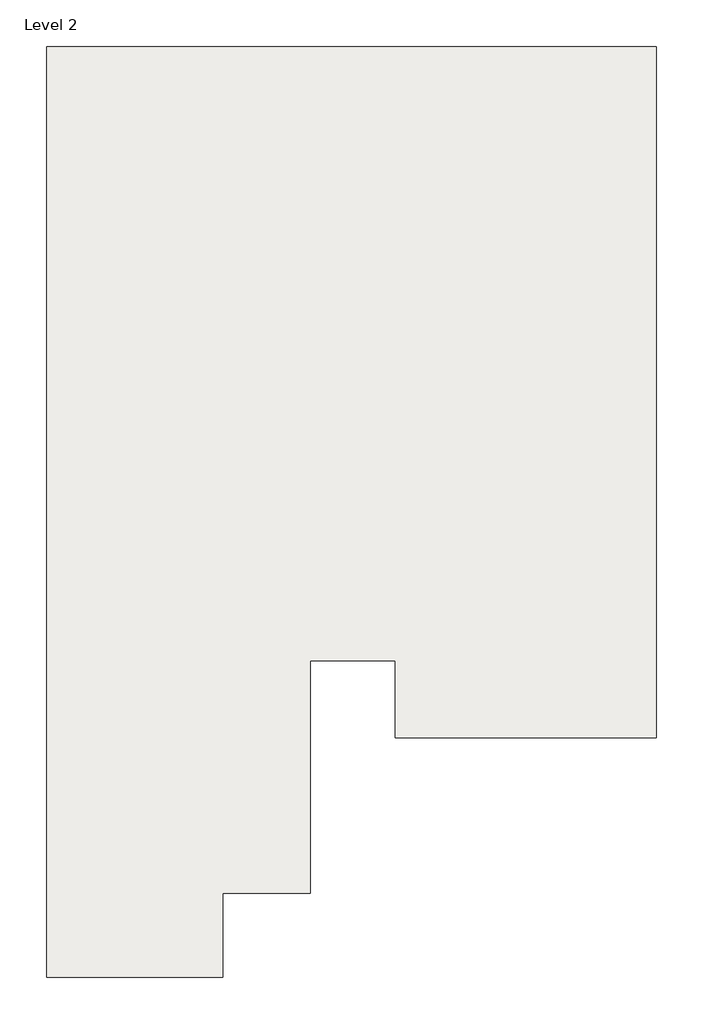
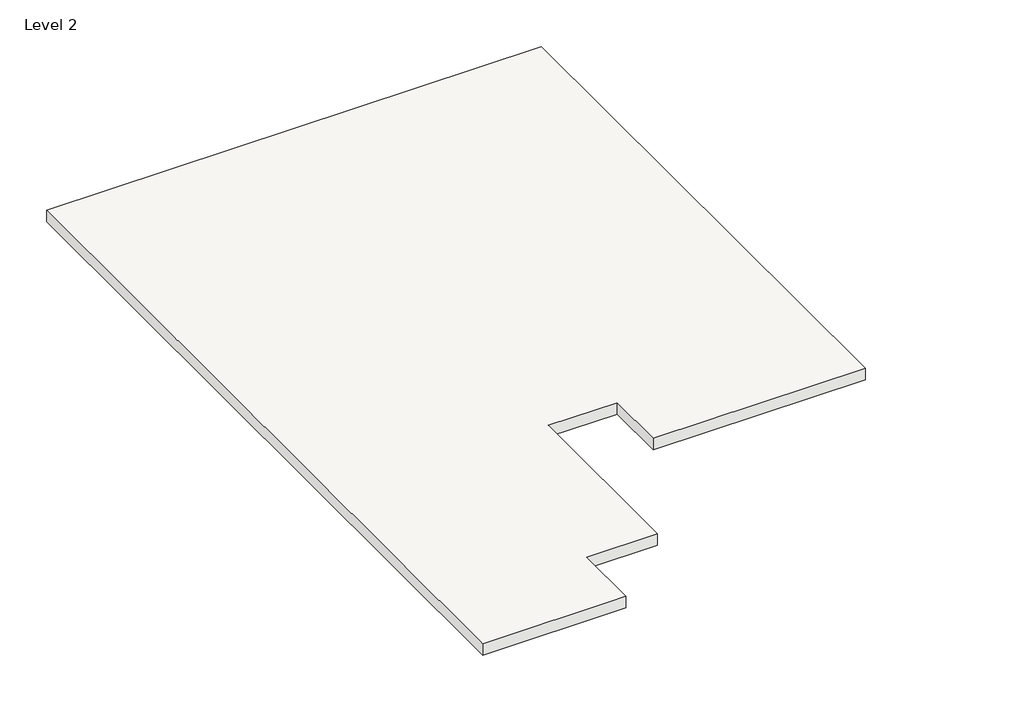
# One storey: 1 roof.
"""IFC4 building model written with IfcOpenShell, lengths in millimetres."""

from ifc_helpers import new_model, si_unit, frame, origin, place, context, project, spatial, polyline, outline, extrude, element, save

model = new_model("IFC4")

# Units and contexts
model_context = context("Model", 3, world=origin())
ifc_project = project(units=[si_unit("LENGTHUNIT", "METRE", prefix="MILLI")], contexts=[model_context])

# Site, building, storey
site = spatial("IfcSite", under=ifc_project)
building = spatial("IfcBuilding", under=site)
storey = spatial("IfcBuildingStorey", under=building, Name="Level 2", Elevation=3048.0)

# Roof
placement = place(None, origin())
element("IfcRoof", 1, ObjectType="Generic - 12\"", at=placement, inside=storey, context=model_context, shape_type="SweptSolid", body=[
    extrude(outline(polyline([(-12134.2789517, 11195.7768478), (260.9210483, 11195.7768478), (260.9210483, -2850.4231522), (-5047.6789517, -2850.4231522), (-5047.6789517, -1287.420591), (-6774.8789517, -1287.420591), (-6774.8789517, -6011.820591), (-8552.8789517, -6011.820591), (-8552.8789517, -7727.2231522), (-12134.2789517, -7727.2231522), (-12134.2789517, 11195.7768478)])), frame((0.0, 0.0, 3048.0), z_axis=(0.0, 0.0, 1.0), x_axis=(1.0, 0.0, 0.0)), (0.0, 0.0, 1.0), 304.8),
])

save(model, "model.ifc")

# Revit data of these elements
# Type "Generic - 12\""
#   Assembly Code = "B1020"
#   Layers, outside or top first: 1' - 0" "Brick, Soldier Course" (function 1)
# Element 1 (IfcRoof, "Generic - 12\"")
#   built-in parameter 1001705 = 11 (stored number, unit not read)
#   built-in parameter 1001710 = 33615
#   Phase Created = New Construction
#   Materials on its faces: "Brick, Soldier Course"
# Materials
#   "Brick, Soldier Course": class "Masonry", colour RGB 170 98 104, transparency 0, Description = "Common brick soldier coursed", Cost = 0
